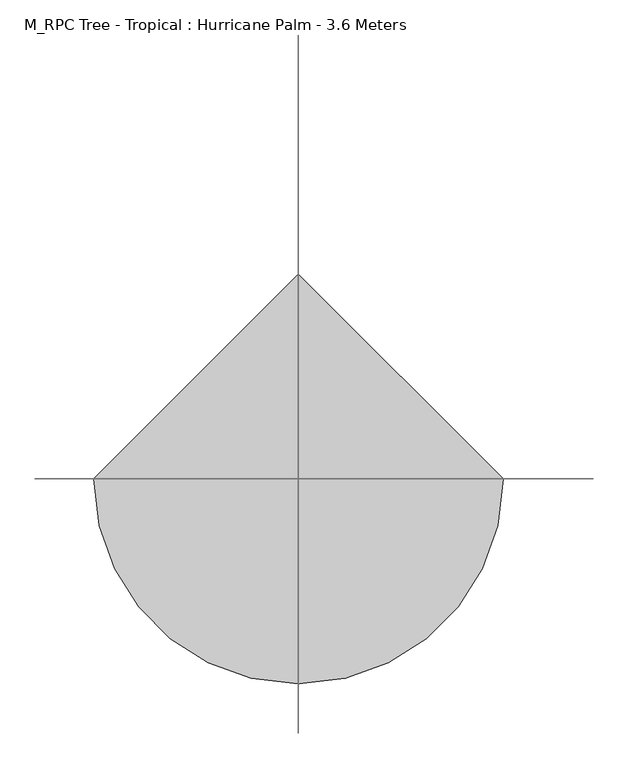
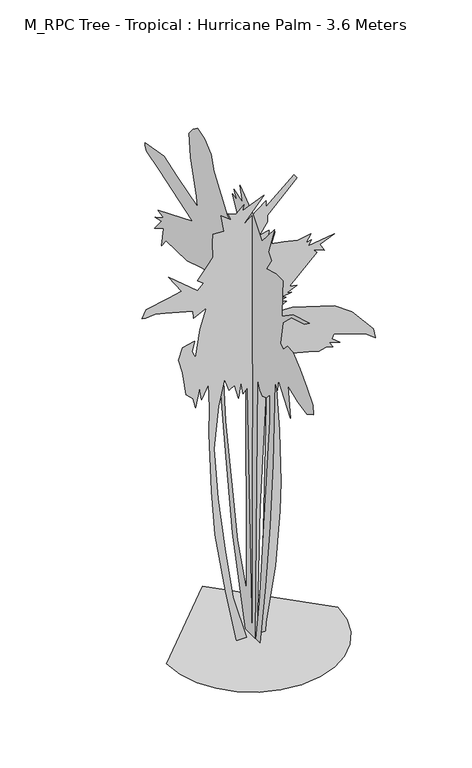
"""IFC4 building model written with IfcOpenShell, lengths in millimetres: geographic element geometry, M_RPC Tree - Tropical : Hurricane Palm - 3.6 Meters."""

from ifc_helpers import new_model, si_unit, origin, place, context, project, spatial, triangles, source, transform, mapped, element, save


def m_rpc_tree_tropical_hurricane_palm_3_6_meters_73a83cb7(model_context):
    return source(origin(), model_context, "Body", "Tessellation", [
        triangles([(-643.5729263, 0.0, 0.0), (-626.5554331, -147.5096553, 0.0), (-578.0829557, -282.9723171, 0.0), (-502.0430114, -402.5097336, 0.0), (-402.3130523, -502.2396927, 0.0), (-282.7756539, -578.2796371, 0.0), (-147.3127378, -626.7520781, 0.0), (0.1966992, -643.7695713, 0.0), (147.7063276, -626.7520781, 0.0), (283.1689802, -578.2796371, 0.0), (402.7064149, -502.2396927, 0.0), (502.436374, -402.5097336, 0.0), (578.4763184, -282.9723171, 0.0), (626.948723, -147.5094101, 0.0), (643.9662163, 5.63e-05, 0.0), (0.1965867, 643.7695713, 0.0), (313.9964953, -0.0001039, 3550.9727875), (336.8464814, -9.66e-05, 3516.6978447), (115.9633523, -6.9e-05, 3299.6230133), (115.9633523, -5.94e-05, 3246.3227783), (55.0301394, -4.68e-05, 3158.7228928), (127.388091, -4.59e-05, 3173.9478355), (123.5800931, -3.79e-05, 3128.2480087), (173.0883084, -3.88e-05, 3147.2980087), (146.4298248, -2.45e-05, 3059.6981232), (237.8295057, -1.72e-05, 3044.4731804), (344.463967, -7e-06, 3017.8230629), (443.4788898, -5.4e-06, 3036.8480644), (405.3964396, 2.9e-06, 2979.7230629), (447.2863973, 3.7e-06, 2987.3481789), (424.4389183, 9.3e-06, 2949.2731773), (618.6612202, 1.44e-05, 2975.9230042), (508.2213407, 1.7e-05, 2930.2231773), (542.4963198, 2.96e-05, 2869.2981171), (458.7138974, 1.92e-05, 2903.5730598), (485.3713546, 2.6e-05, 2873.0981758), (279.7214799, 5.1e-05, 2675.0733444), (336.8464814, 5.6e-05, 2663.6481697), (260.6790012, 5.75e-05, 2633.1732857), (294.9539804, 6.06e-05, 2625.5734589), (222.5965147, 5.9e-05, 2614.1482841), (253.0640046, 6.33e-05, 2598.8983429), (203.5545266, 6.35e-05, 2583.6734001), (256.8714938, 6.96e-05, 2564.6234001), (138.8133293, 7.38e-05, 2507.4983986), (302.571466, 8.28e-05, 2503.6983398), (618.6612202, 0.0001165, 2404.6785118), (748.1461945, 0.0001401, 2309.4709511), (911.9035681, 0.0001824, 2119.0536495), (927.1360685, 0.0001975, 2039.0787346), (862.3961248, 0.0001847, 2092.3961197), (614.8537491, 0.0001558, 2183.796064), (599.621285, 0.0001612, 2149.5211212), (660.5537212, 0.0001731, 2100.0112072), (580.5788063, 0.000165, 2122.8611206), (607.2362998, 0.0001738, 2080.9712357), (553.9213128, 0.0001684, 2096.2035908), (500.603855, 0.0001677, 2084.7787067), (424.4389183, 0.0001605, 2103.8211491), (294.9539804, 0.0001478, 2138.0960918), (165.4715495, 0.0001324, 2187.6035351), (203.5545266, 0.0002474, 1555.4214832), (214.979774, 0.0003208, 1147.9292776), (207.3630332, 0.0003613, 919.4294168), (176.8963064, 0.000436, 492.897167), (104.5381049, 0.0005079, 70.1739552), (100.7298617, 0.0005209, 0.0040319), (55.0301394, 0.0005192, 6.64e-05), (85.4966164, 0.0003735, 816.6069866), (115.9633523, 0.0001415, 2122.8611206), (58.8383826, 0.0003408, 991.7893896), (35.9881467, 0.0005174, 0.0040343), (1.7132677, 0.0005156, 0.0040356), (-36.3698072, 0.000159, 1981.9537331), (-70.644784, 0.000164, 1943.8713192), (-85.8780248, 0.0001456, 2042.8862057), (-101.1115154, 0.0001666, 1921.0212605), (-131.5782422, 0.0001446, 2035.2712635), (-173.4697168, 0.0001473, 2008.6112629), (-207.7446959, 0.0001278, 2107.6286201), (-253.4456673, 0.0001609, 1909.5962311), (-287.7181575, 0.0002171, 1585.8889549), (-257.2531747, 0.0002915, 1178.3967493), (-203.9362075, 0.0003691, 759.4819851), (-143.00299, 0.0004443, 355.7972869), (-43.9865502, 0.0005125, 0.0080045), (-116.3447516, 0.0005097, 0.00404), (-200.1279552, 0.0004299, 420.5397377), (-280.1031608, 0.00034, 900.3894453), (-306.7606361, 0.0002753, 1254.5642658), (-325.8031148, 0.000192, 1715.3714584), (-321.9931003, 0.0001554, 1921.0212605), (-329.6106222, 0.000121, 2111.4360912), (-379.1180655, 0.0001375, 2004.8036465), (-394.353073, 0.000119, 2103.8211491), (-424.8205447, 0.0001434, 1959.1036743), (-443.8605526, 0.0001288, 2035.2712635), (-497.1780104, 0.0001172, 2084.7787067), (-523.8354675, 8.25e-05, 2271.3860664), (-554.3029756, 6.12e-05, 2381.8284531), (-523.8354675, 4.71e-05, 2469.4184555), (-432.4355596, 4.83e-05, 2488.4608978), (-451.4780382, 6.1e-05, 2412.293454), (-424.8205447, 7.26e-05, 2355.1709232), (-390.5430585, 3.62e-05, 2568.4234589), (-344.8430863, 1.06e-05, 2724.57323), (-440.0530452, 1.46e-05, 2675.0733444), (-443.8605526, 4.2e-06, 2732.1983459), (-653.317971, -1.66e-05, 2789.3233475), (-729.4854149, -2.39e-05, 2808.3480583), (-801.8428442, -2.62e-05, 2800.7482315), (-828.5028448, -2.89e-05, 2808.3480583), (-798.0353731, -3.76e-05, 2865.4730598), (-630.467985, -3.52e-05, 2899.7480026), (-531.4529895, -3.43e-05, 2922.5980614), (-630.467985, -6.52e-05, 3067.3229485), (-409.5855735, -2.06e-05, 2880.7232918), (-367.6930724, -2.67e-05, 2926.4231186), (-409.5855735, -3.49e-05, 2960.6980614), (-337.2281078, -4.83e-05, 3055.8980644), (-295.3356431, -5.57e-05, 3109.2230072), (-299.1456395, -7.63e-05, 3223.4730103), (-295.3356431, -8.84e-05, 3292.0228958), (-211.5526939, -8.28e-05, 3284.3977798), (-234.4029343, -0.0001078, 3417.6977829), (-158.2362353, -9.3e-05, 3356.7477242), (-181.0864758, -0.0001044, 3413.8727257), (-120.1530039, -9.66e-05, 3387.2228989), (-63.0282885, -0.0001039, 3444.3479004), (-74.4530318, -9.63e-05, 3398.6477829), (89.305114, -0.0001003, 3467.1976685), (-74.4530318, -7.52e-05, 3280.5980118), (104.5381049, -9.06e-05, 3417.6977829), (104.5381049, -8.18e-05, 3368.1728989), (0.1966746, 109.7849322, 2058.8987457), (0.1966737, 136.4211607, 1982.7937981), (0.1966621, 178.2778899, 2203.4960243), (0.1966558, 208.7196183, 2294.8185024), (0.1966526, 254.3823289, 2218.7160255), (0.1966467, 322.8748052, 2142.6110779), (0.1966388, 398.9797528, 2104.5612202), (0.1966634, 345.7072778, 1491.9265217), (0.1967073, 189.6938719, 643.3695957), (0.1967308, 75.5382035, 312.3198172), (0.196676, 83.1486947, 2119.781076), (0.196648, 711.0045662, 3599.997702), (0.1966593, 623.4846176, 3569.5478165), (0.1966719, 535.964669, 3497.2478691), (0.196679, 501.7196663, 3394.522744), (0.1966946, 406.5897534, 3253.722908), (0.1967081, 322.8748052, 3135.7731308), (0.1967188, 242.9660926, 3093.8980705), (0.1967273, 155.4471432, 3158.5979004), (0.1967093, 258.1873292, 3352.6729729), (0.196717, 197.3038725, 3337.4477394), (0.1967102, 239.1608379, 3398.3228027), (0.1967248, 125.005424, 3364.0728584), (0.1967173, 159.2518892, 3482.0476341), (0.1967415, -11.9810172, 3352.6729729), (0.1967594, -126.1366685, 3208.0730782), (0.1967733, -289.7598207, 3398.3228027), (0.1967703, -209.8506176, 3177.6229019), (0.1967768, -251.7073468, 3128.1480148), (0.1967717, -183.21438, 3025.4231804), (0.1967856, -308.7847858, 3059.6731247), (0.1967965, -400.1097347, 3059.6731247), (0.1967989, -392.4997341, 2949.3231743), (0.1968038, -388.6947338, 2770.4733353), (0.1968176, -529.4871574, 2869.398111), (0.1968412, -742.5770576, 2930.2731743), (0.1968353, -681.694582, 2884.6230537), (0.1968168, -514.2646854, 2835.1481667), (0.1968064, -400.1097347, 2728.598275), (0.1968079, -365.8622612, 2542.1483185), (0.1968131, -403.914735, 2519.3232582), (0.1968177, -457.1872101, 2576.3982628), (0.1968265, -529.4871574, 2572.5984947), (0.1968401, -624.6146358, 2496.4935471), (0.1968533, -712.1345118, 2401.3659233), (0.1968656, -792.0444597, 2310.0409744), (0.1968686, -799.6544603, 2237.7410271), (0.1968597, -712.1345118, 2188.2735523), (0.1968448, -594.1746334, 2214.9110252), (0.1968283, -468.602211, 2268.1835003), (0.1968387, -495.2396839, 2024.6512722), (0.1968143, -343.0322957, 2233.9360268), (0.1968151, -327.8122945, 2146.4186943), (0.1968101, -297.3698031, 2192.0785526), (0.1968268, -270.7323302, 1526.1715244), (0.1968377, -232.6816004, 1008.6668478), (0.1968461, -175.6038889, 498.7721718), (0.1968523, -103.3054313, 0.0065168), (0.1968459, -50.03272, 0.0065184), (0.1968415, -91.8899398, 316.1247811), (0.1968127, -232.6816004, 1845.8088455), (0.1968065, -232.6816004, 2055.0937454), (0.1968026, -187.0193803, 2001.8212704), (0.1967969, -133.7469144, 1982.7937981), (0.196792, -99.5001857, 2009.431271), (0.1967862, -69.0587072, 2081.7286022), (0.1968445, -38.6169743, 0.0104859), (0.1968297, 86.9539402, 0.0065225), (0.1967899, 254.3823289, 662.3945972), (0.1967589, 357.1222787, 1294.0566227), (0.1967248, 456.0571918, 2039.8711281), (0.1967207, 456.0571918, 2180.6635517), (0.1967161, 505.5246666, 2135.0010773), (0.1967156, 459.8621922, 2336.6759766), (0.1967101, 501.7196663, 2351.8984486), (0.1967089, 478.8871937, 2485.0785461), (0.1967046, 520.7446678, 2462.2485443), (0.1967001, 535.964669, 2549.7734344), (0.1966864, 657.7320911, 2523.123317), (0.1966655, 847.9894461, 2462.2485443), (0.1966331, 1121.9642927, 2454.6385437), (0.1966285, 1179.0417681, 2382.338451), (0.1966272, 1152.4042952, 2530.7484329), (0.1966151, 1270.3666443, 2466.0535446), (0.1966227, 1179.0417681, 2576.3982628), (0.1966133, 1262.7566437, 2557.3732613), (0.1966241, 1156.2117662, 2618.2483246), (0.1966154, 1224.7041698, 2637.2983246), (0.1966631, 779.4969698, 2819.9232239), (0.196607, 1213.2892416, 2964.5231186), (0.1965862, 1376.9115944, 3010.1979469), (0.1965829, 1395.9365959, 3044.4481819), (0.1965822, 1395.9365959, 3067.2729515), (0.1966104, 1148.5992949, 3109.1230133), (0.1966334, 969.7568682, 3052.0480087), (0.1966662, 714.8095665, 2972.1482346), (0.1966629, 722.4195671, 3052.0480087), (0.1966456, 802.3295151, 3314.5979713), (0.196638, 821.3544439, 3493.4478104), (0.1966421, 771.8870419, 3554.3475815), (0.1967197, 29.876231, 2180.6635517), (0.1967832, 3.2397229, 156.3063931), (0.1967254, -11.9809423, 2157.8335499)], [[15, 16, 1], [14, 15, 1], [14, 1, 2], [13, 14, 2], [13, 2, 3], [13, 3, 4], [12, 13, 4], [11, 12, 4], [11, 4, 5], [11, 5, 6], [11, 6, 7], [11, 7, 8], [11, 8, 9], [11, 9, 10], [31, 32, 33], [115, 116, 117], [39, 40, 41], [76, 77, 78], [53, 54, 55], [95, 96, 97], [130, 131, 132], [128, 129, 130], [37, 38, 39], [93, 94, 95], [33, 34, 35], [49, 50, 51], [31, 33, 35], [55, 56, 57], [124, 125, 126], [41, 42, 43], [126, 127, 128], [27, 28, 29], [43, 44, 45], [29, 30, 31], [74, 75, 76], [23, 24, 25], [132, 133, 134], [101, 102, 103], [106, 107, 108], [100, 101, 103], [21, 22, 23], [128, 130, 132], [126, 128, 132], [78, 79, 80], [85, 86, 87], [85, 87, 88], [84, 85, 88], [84, 88, 89], [83, 84, 89], [83, 89, 90], [82, 83, 90], [82, 90, 91], [81, 82, 91], [81, 91, 92], [48, 49, 51], [48, 51, 52], [111, 112, 113], [47, 48, 52], [110, 111, 113], [110, 113, 114], [109, 110, 114], [134, 17, 18], [134, 18, 19], [132, 134, 19], [95, 97, 98], [67, 68, 69], [66, 67, 69], [65, 66, 69], [64, 65, 69], [64, 69, 70], [63, 64, 70], [62, 63, 70], [61, 62, 70], [124, 126, 132], [132, 19, 20], [132, 20, 21], [95, 98, 99], [122, 123, 124], [99, 100, 103], [99, 103, 104], [72, 73, 74], [71, 72, 74], [70, 71, 74], [70, 74, 76], [118, 119, 120], [95, 99, 104], [93, 95, 104], [35, 36, 37], [80, 81, 92], [80, 92, 93], [108, 109, 114], [108, 114, 115], [108, 115, 117], [106, 108, 117], [31, 35, 37], [46, 47, 52], [46, 52, 53], [46, 53, 55], [46, 55, 57], [46, 57, 58], [46, 58, 59], [46, 59, 60], [46, 60, 61], [45, 46, 61], [80, 93, 104], [106, 117, 118], [29, 31, 37], [27, 29, 37], [26, 27, 37], [25, 26, 37], [121, 122, 124], [121, 124, 132], [121, 132, 21], [76, 78, 80], [80, 104, 105], [70, 76, 80], [70, 80, 105], [61, 70, 105], [45, 61, 105], [45, 105, 106], [43, 45, 106], [41, 43, 106], [41, 106, 118], [41, 118, 120], [41, 120, 121], [41, 121, 21], [41, 21, 23], [41, 23, 25], [41, 25, 37], [41, 37, 39], [235, 144, 145], [144, 235, 236], [219, 220, 221], [160, 161, 162], [169, 170, 171], [169, 171, 172], [217, 218, 219], [215, 216, 217], [184, 185, 186], [135, 136, 137], [168, 169, 172], [168, 172, 173], [206, 207, 208], [157, 158, 159], [221, 222, 223], [155, 156, 157], [186, 187, 188], [145, 135, 146], [145, 146, 147], [145, 147, 148], [145, 148, 149], [145, 149, 150], [145, 150, 151], [153, 154, 155], [145, 151, 152], [235, 145, 152], [210, 211, 212], [192, 193, 194], [191, 192, 194], [191, 194, 195], [190, 191, 195], [189, 190, 195], [188, 189, 195], [188, 195, 196], [165, 166, 167], [153, 155, 157], [153, 157, 159], [153, 159, 160], [226, 227, 228], [225, 226, 228], [224, 225, 228], [223, 224, 228], [223, 228, 229], [223, 229, 230], [208, 209, 210], [201, 202, 203], [162, 163, 164], [160, 162, 164], [153, 160, 164], [214, 215, 217], [164, 165, 167], [164, 167, 168], [235, 152, 153], [235, 153, 164], [235, 164, 168], [235, 168, 173], [235, 173, 174], [237, 235, 174], [237, 174, 175], [180, 181, 182], [179, 180, 182], [179, 182, 183], [179, 183, 184], [178, 179, 184], [177, 178, 184], [176, 177, 184], [175, 176, 184], [237, 175, 184], [237, 184, 186], [237, 186, 188], [237, 188, 196], [237, 196, 197], [217, 219, 221], [214, 217, 221], [214, 221, 223], [213, 214, 223], [212, 213, 223], [212, 223, 230], [197, 198, 199], [197, 199, 200], [237, 197, 200], [236, 237, 200], [236, 200, 201], [236, 201, 203], [144, 236, 203], [143, 144, 203], [142, 143, 203], [142, 203, 204], [142, 204, 205], [141, 142, 205], [141, 205, 206], [140, 141, 206], [140, 206, 208], [139, 140, 208], [138, 139, 208], [138, 208, 210], [232, 233, 234], [232, 234, 146], [231, 232, 146], [210, 212, 230], [138, 210, 230], [138, 230, 231], [138, 231, 146], [138, 146, 135], [138, 135, 137]], closed=False),
    ])


if __name__ == "__main__":
    model = new_model("IFC4")
    model_context = context("Model", 3, world=origin())
    ifc_project = project(units=[si_unit("LENGTHUNIT", "METRE", prefix="MILLI")], contexts=[model_context])
    site = spatial("IfcSite", under=ifc_project)
    building = spatial("IfcBuilding", under=site)
    placement = place(None, origin())
    m_rpc_tree_tropical_hurricane_palm_3_6_meters_shape = m_rpc_tree_tropical_hurricane_palm_3_6_meters_73a83cb7(model_context)
    element("IfcGeographicElement", 1, ObjectType="M_RPC Tree - Tropical : Hurricane Palm - 3.6 Meters", at=placement, inside=building, context=model_context, shape_type="MappedRepresentation", body=[
        mapped(m_rpc_tree_tropical_hurricane_palm_3_6_meters_shape, transform((0.0, 0.0, 0.0), x_axis=(1.0, 0.0, 0.0), y_axis=(0.0, 1.0, 0.0), z_axis=(0.0, 0.0, 1.0))),
    ])
    save(model, "model.ifc")

# Revit data of these elements
# Type "M_RPC Tree - Tropical : Hurricane Palm - 3.6 Meters"
#   built-in parameter 1005198 = "{2, 15},{39, RPC-16-FXGL-UL7X-PH44-0000-ST1L-LVER-AU},{1, 0},{1, 0},{2, 35},{1, 8},{5, Color},{1, 0},{1, 0},{3, 0.8},{3, 0.8},{3, 0.8},{1, 8},{7, BBoxMin},{1, 0},{1, 0},{1, 0},{1, 0},{1, 0},{1, 8},{7, BBoxMax},{1, 0},{1, 0},{1, 0},{1, 0},{1, 0},{2, 11},{9, RPCTypeId},{1, 0},{1, 0},{39, RPC-16-FXGL-UL7X-PH44-0000-ST1L-LVER-AU},{1, 6},{14, RPCPlantHeight},{1, 0},{1, 0},{6, 11.811},{2, 11},{7, keyword},{1, 0},{1, 0},{102, :Geometry:RPC:Hurricane Palm:Ptychosperma macarthurii (New Guinea):with jagged leaftips:palm:tropical.},{2, 11},{8, category},{1, 0},{1, 0},{17, :Trees [Tropical]},{2, 11},{12, LocalizedUID},{1, 0},{1, 0},{14, Hurricane Palm},{2, 14},{6, Height},{1, 0},{1, 0},{6, 11.811},{1, 2},{16, Cast Reflections},{1, 0},{1, 0},{1, 0},{1, 2},{12, Cast Shadows},{1, 0},{1, 0},{1, 1},{1, 2},{9, Lock View},{1, 0},{1, 0},{1, 0},{1, 4},{5, ViewC},{1, 0},{1, 0},{1, 0},{2, 11},{20, AdvancedUIDefinition},{1, 0},{1, 0},{0, },{2, 11},{10, AssetLibID},{1, 0},{1, 0},{36, 4D3F6E72-3F99-4203-98E9-AF80B3C7A7A4},{2, 11},{10, BaseSchema},{1, 0},{1, 0},{9, RPCSchema},{2, 11},{12, ExchangeGUID},{1, 0},{1, 0},{0, },{1, 2},{6, Hidden},{1, 0},{1, 0},{1, 0},{1, 4},{11, RPCCategory},{1, 0},{1, 0},{1, 0},{2, 11},{8, RPCImage},{1, 0},{1, 0},{0, },{1, 4},{13, SchemaVersion},{1, 0},{1, 0},{1, 4},{2, 11},{12, UIDefinition},{1, 0},{1, 0},{0, },{2, 11},{6, UIName},{1, 0},{1, 0},{39, RPC-16-FXGL-UL7X-PH44-0000-ST1L-LVER-AU},{2, 11},{11, VersionGUID},{1, 0},{1, 0},{9, RPCSchema},{2, 11},{9, assettype},{1, 0},{1, 0},{11, RPCGeometry},{2, 11},{11, description},{1, 0},{1, 0},{0, },{2, 11},{9, localname},{1, 0},{1, 0},{3, RPC},{2, 11},{9, localtype},{1, 0},{1, 0},{3, RPC},{1, 4},{8, revision},{1, 0},{1, 0},{1, 1},{2, 11},{9, thumbnail},{1, 0},{1, 0},{0, },{1, 4},{7, version},{1, 0},{1, 0},{1, 1},{1, 2},{20, RPC_Cast Reflections},{1, 0},{1, 0},{1, 1},{1, 2},{16, RPC_Cast Shadows},{1, 0},{1, 0},{1, 1},{1, 2},{13, RPC_Lock View},{1, 0},{1, 0},{1, 0},{1, 4},{9, RPC_ViewC},{1, 0},{1, 0},{1, 0},{21, assetlibrary_base.fbx},{1, 5},"
#   built-in parameter 1005195 = "RPC-16-FXGL-UL7X-PH44-0000-ST1L-LVER-AU"
#   Type Comments = "Hurricane Palm"
#   Height = 3600 mm
#   Plan Symbol = element 405753
#   Description = (empty or 0)
#   Default Elevation = 0
